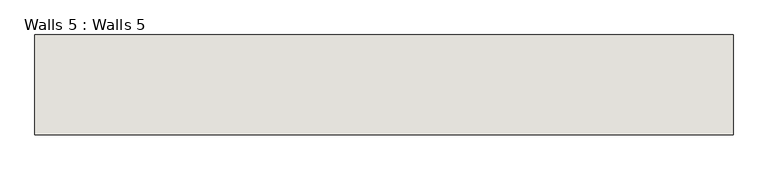
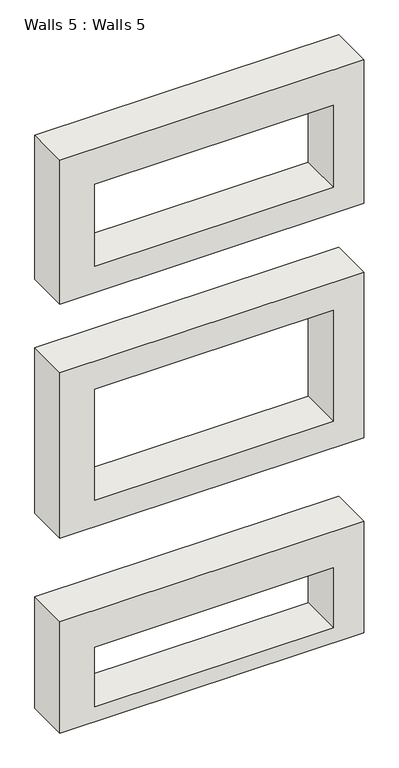
"""IFC4 building model written with IfcOpenShell, lengths in millimetres: wall geometry, Walls 5 : Walls 5."""

from ifc_helpers import new_model, si_unit, frame, origin, place, context, project, spatial, polyline, outline, extrude, source, transform, mapped, element, save


def walls_5_walls_5_99fd860d(model_context):
    return source(origin(), model_context, "Body", "SweptSolid", [
        extrude(outline(polyline([(4625.037369, -10173.2352914), (4625.037369, -12306.8352914), (3558.237369, -12306.8352914), (3558.237369, -10173.2352914), (4625.037369, -10173.2352914)]), holes=[polyline([(4361.8557587, -10385.6641524), (3752.2557587, -10385.6641524), (3752.2557587, -12062.0641524), (4361.8557587, -12062.0641524), (4361.8557587, -10385.6641524)])]), frame((0.0, -20740.5210337, 0.0), z_axis=(0.0, 1.0, 0.0), x_axis=(0.0, 0.0, 1.0)), (0.0, 0.0, 1.0), 304.8),
        extrude(outline(polyline([(3048.0, -10173.2352914), (3048.0, -12306.8352914), (1819.3944812, -12306.8352914), (1819.3944812, -10173.2352914), (3048.0, -10173.2352914)]), holes=[polyline([(2838.5056331, -10385.6641524), (2015.7072574, -10385.6641524), (2015.7072574, -12062.0641524), (2838.5056331, -12062.0641524), (2838.5056331, -10385.6641524)])]), frame((0.0, -20740.5210337, 0.0), z_axis=(0.0, 1.0, 0.0), x_axis=(0.0, 0.0, 1.0)), (0.0, 0.0, 1.0), 304.8),
        extrude(outline(polyline([(1198.7914462, -10173.2352914), (1198.7914462, -12306.8352914), (371.3207327, -12306.8352914), (371.3207327, -10173.2352914), (1198.7914462, -10173.2352914)]), holes=[polyline([(924.8790164, -10385.6641524), (482.8177328, -10385.6641524), (482.8177328, -12062.0641524), (924.8790164, -12062.0641524), (924.8790164, -10385.6641524)])]), frame((0.0, -20740.5210337, 0.0), z_axis=(0.0, 1.0, 0.0), x_axis=(0.0, 0.0, 1.0)), (0.0, 0.0, 1.0), 304.8),
    ])


if __name__ == "__main__":
    model = new_model("IFC4")
    model_context = context("Model", 3, world=origin())
    ifc_project = project(units=[si_unit("LENGTHUNIT", "METRE", prefix="MILLI")], contexts=[model_context])
    site = spatial("IfcSite", under=ifc_project)
    building = spatial("IfcBuilding", under=site)
    placement = place(None, origin())
    walls_5_walls_5_shape = walls_5_walls_5_99fd860d(model_context)
    element("IfcWall", 1, ObjectType="Walls 5 : Walls 5", at=placement, inside=building, context=model_context, shape_type="MappedRepresentation", body=[
        mapped(walls_5_walls_5_shape, transform((0.0, 0.0, 0.0), x_axis=(1.0, 0.0, 0.0), y_axis=(0.0, 1.0, 0.0), z_axis=(0.0, 0.0, 1.0))),
    ])
    save(model, "model.ifc")

# Revit data of these elements
# Element 1 (IfcWall, "Walls 5 : Walls 5")
#   Materials on its faces: "Default Wall"
# Materials
#   "Default Wall": colour RGB 80 80 80, transparency 0
